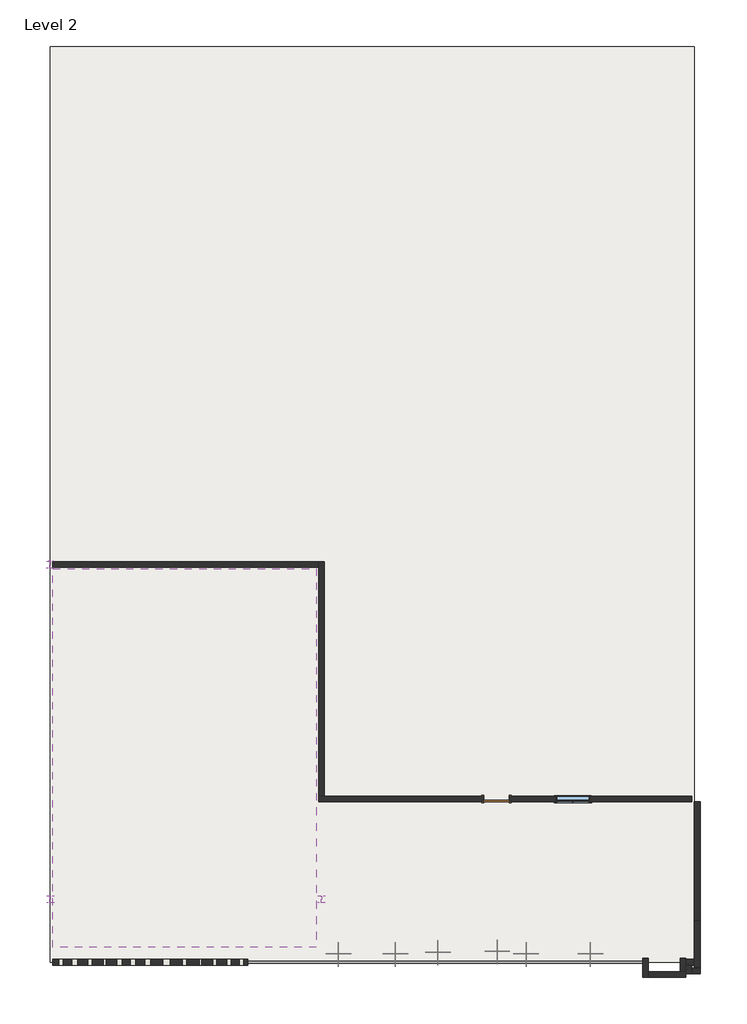
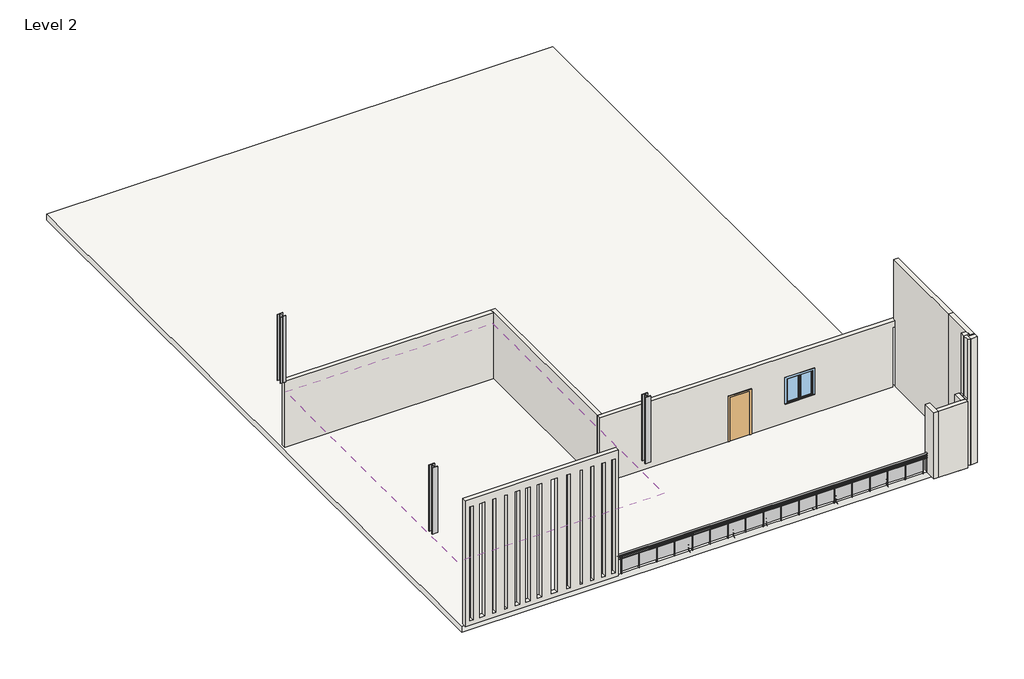
# One storey: 14 walls, 6 geographic elements, 3 columns, 1 covering, 1 door, 1 railing, 1 slab, 1 window.
"""IFC4 building model written with IfcOpenShell, lengths in millimetres."""

from ifc_helpers import new_model, si_unit, point, frame, origin, place, context, project, spatial, polyline, ellipse_curve, trimmed, outline, extrude, faceted_brep, transform, mapped, element, save
from ifc_brep_helpers import plane_surface, extruded_surface, advanced_brep
from components import w_shapes_column_w10x49_28d960f7, door_54dd4da4, rpc_plant_tropical_agave_1_5_93a2a214, window_0862ab64

model = new_model("IFC4")

# Units and contexts
model_context = context("Model", 3, world=origin())
ifc_project = project(units=[si_unit("LENGTHUNIT", "METRE", prefix="MILLI")], contexts=[model_context])

# Site, building, storey
site = spatial("IfcSite", under=ifc_project)
building = spatial("IfcBuilding", under=site)
storey = spatial("IfcBuildingStorey", under=building, Name="Level 2", Elevation=3200.4)

# Columns
placement = place(None, origin())
w_shapes_column_w10x49_shape = w_shapes_column_w10x49_28d960f7(model_context)
element("IfcColumn", 1, ObjectType="W Shapes-Column : W10X49", at=placement, inside=storey, context=model_context, shape_type="MappedRepresentation", body=[
    mapped(w_shapes_column_w10x49_shape, transform((-18401.1950104, -14607.7898918, 0.0), x_axis=(1.0, 0.0, 0.0), y_axis=(0.0, 1.0, 0.0), z_axis=(0.0, 0.0, 1.0))),
])
element("IfcColumn", 2, ObjectType="W Shapes-Column : W10X49", at=placement, inside=storey, context=model_context, shape_type="MappedRepresentation", body=[
    mapped(w_shapes_column_w10x49_shape, transform((-18401.1950104, -2573.393541, 0.0), x_axis=(1.0, 0.0, 0.0), y_axis=(0.0, 1.0, 0.0), z_axis=(0.0, 0.0, 1.0))),
])
element("IfcColumn", 3, ObjectType="W Shapes-Column : W10X49", at=placement, inside=storey, context=model_context, shape_type="MappedRepresentation", body=[
    mapped(w_shapes_column_w10x49_shape, transform((-8647.5950104, -14607.7898918, 0.0), x_axis=(1.0, 0.0, 0.0), y_axis=(0.0, 1.0, 0.0), z_axis=(0.0, 0.0, 1.0))),
])

# Covering
element("IfcCovering", 4, ObjectType="2' x 4' ACT System", at=placement, inside=storey, context=model_context, shape_type="SweptSolid", body=[
    extrude(outline(polyline([(-8829.5340594, -2725.793541), (-8829.5340594, -11305.7898918), (-8829.5340594, -16334.9898918), (-18299.5950104, -16334.9898918), (-18299.5950104, -2725.793541), (-8829.5340594, -2725.793541)])), frame((0.0, 0.0, 5943.6), z_axis=(0.0, 0.0, 1.0), x_axis=(1.0, 0.0, 0.0)), (0.0, 0.0, 1.0), 57.15),
    extrude(outline(polyline([(4712.8049896, -11305.7898918), (4712.8049896, -16334.9898918), (-8545.9950104, -16334.9898918), (-8545.9950104, -11305.7898918), (4712.8049896, -11305.7898918)])), frame((0.0, 0.0, 5943.6), z_axis=(0.0, 0.0, 1.0), x_axis=(1.0, 0.0, 0.0)), (0.0, 0.0, 1.0), 57.15),
])

# Door
door_shape = door_54dd4da4(model_context)
element("IfcDoor", 5, ObjectType="Single-Flush : 36\" x 84\"", at=placement, inside=storey, context=model_context, shape_type="MappedRepresentation", body=[
    mapped(door_shape, transform((-2348.3950104, -11000.9898918, 3200.4), x_axis=(-1.0, 0.0, 0.0), y_axis=(0.0, -1.0, 0.0), z_axis=(0.0, 0.0, 1.0))),
])

# Geographic elements
rpc_plant_tropical_agave_1_5_shape = rpc_plant_tropical_agave_1_5_93a2a214(model_context)
element("IfcGeographicElement", 6, ObjectType="RPC Plant - Tropical : Agave - 1.5'", at=placement, inside=storey, context=model_context, shape_type="MappedRepresentation", body=[
    mapped(rpc_plant_tropical_agave_1_5_shape, transform((-8037.9950104, -16571.4958521, 3200.4), x_axis=(1.0, 0.0, 0.0), y_axis=(0.0, 1.0, 0.0), z_axis=(0.0, 0.0, 1.0))),
])
element("IfcGeographicElement", 7, ObjectType="RPC Plant - Tropical : Agave - 1.5'", at=placement, inside=storey, context=model_context, shape_type="MappedRepresentation", body=[
    mapped(rpc_plant_tropical_agave_1_5_shape, transform((1023.9459392, -16571.4958521, 3200.4), x_axis=(1.0, 0.0, 0.0), y_axis=(0.0, 1.0, 0.0), z_axis=(0.0, 0.0, 1.0))),
])
element("IfcGeographicElement", 8, ObjectType="RPC Plant - Tropical : Agave - 1.5'", at=placement, inside=storey, context=model_context, shape_type="MappedRepresentation", body=[
    mapped(rpc_plant_tropical_agave_1_5_shape, transform((-1287.4540608, -16571.4958521, 3200.4), x_axis=(1.0, 0.0, 0.0), y_axis=(0.0, 1.0, 0.0), z_axis=(0.0, 0.0, 1.0))),
])
element("IfcGeographicElement", 9, ObjectType="RPC Plant - Tropical : Agave - 1.5'", at=placement, inside=storey, context=model_context, shape_type="MappedRepresentation", body=[
    mapped(rpc_plant_tropical_agave_1_5_shape, transform((-4462.4540608, -16512.2981542, 3200.4), x_axis=(1.0, 0.0, 0.0), y_axis=(0.0, 1.0, 0.0), z_axis=(0.0, 0.0, 1.0))),
])
element("IfcGeographicElement", 10, ObjectType="RPC Plant - Tropical : Agave - 1.5'", at=placement, inside=storey, context=model_context, shape_type="MappedRepresentation", body=[
    mapped(rpc_plant_tropical_agave_1_5_shape, transform((-5986.4540608, -16571.4958521, 3200.4), x_axis=(1.0, 0.0, 0.0), y_axis=(0.0, 1.0, 0.0), z_axis=(0.0, 0.0, 1.0))),
])
element("IfcGeographicElement", 11, ObjectType="RPC Plant - Tropical : Agave - 1.5'", at=placement, inside=storey, context=model_context, shape_type="MappedRepresentation", body=[
    mapped(rpc_plant_tropical_agave_1_5_shape, transform((-2328.8540608, -16476.9736509, 3200.4), x_axis=(1.0, 0.0, 0.0), y_axis=(0.0, 1.0, 0.0), z_axis=(0.0, 0.0, 1.0))),
])

# Railing
element("IfcRailing", 12, ObjectType="Glass Panel - Bottom Fill", at=placement, inside=storey, context=model_context, shape_type="SolidModel", body=[
    advanced_brep(
    [(-11289.1950104, -16830.2898918, 4114.8), (-11289.1950104, -16906.4898918, 4114.8), (2903.5459392, -16830.2898918, 4114.8), (2903.5459392, -16906.4898918, 4114.8)],
    [
        (0, 1, ellipse_curve(frame((-11289.1950104, -16868.3898918, 4114.8), z_axis=(-1.0, 0.0, 0.0), x_axis=(0.0, -1.0, 0.0)), 38.1, 28.575)),
        (1, 0, ellipse_curve(frame((-11289.1950104, -16868.3898918, 4114.8), z_axis=(-1.0, 0.0, 0.0), x_axis=(0.0, -1.0, 0.0)), 38.1, 28.575)),
        (2, 3, ellipse_curve(frame((2903.5459392, -16868.3898918, 4114.8), z_axis=(1.0, 0.0, 0.0), x_axis=(0.0, -1.0, 0.0)), 38.1, 28.575)),
        (3, 2, ellipse_curve(frame((2903.5459392, -16868.3898918, 4114.8), z_axis=(1.0, 0.0, 0.0), x_axis=(0.0, -1.0, 0.0)), 38.1, 28.575)),
        (0, 2),
        (3, 1),
    ],
    [
        plane_surface(frame((-11289.1950104, -16868.3898918, 4114.8), z_axis=(-1.0, 0.0, 0.0), x_axis=(0.0, 1.0, 0.0))),
        plane_surface(frame((2903.5459392, -16868.3898918, 4114.8), z_axis=(1.0, 0.0, 0.0), x_axis=(0.0, 1.0, 0.0))),
        extruded_surface(trimmed(ellipse_curve(frame((2903.5459392, -16868.3898918, 4114.8), z_axis=(-1.0, 0.0, 0.0), x_axis=(0.0, -1.0, 0.0)), 38.1, 28.575), [point((2903.5459392, -16830.2898918, 4114.8))], [point((2903.5459392, -16906.4898918, 4114.8))], True, "CARTESIAN"), (-14192.7409496, 0.0, 0.0), 14192.7409496),
        extruded_surface(trimmed(ellipse_curve(frame((2903.5459392, -16868.3898918, 4114.8), z_axis=(-1.0, 0.0, 0.0), x_axis=(0.0, -1.0, 0.0)), 38.1, 28.575), [point((2903.5459392, -16906.4898918, 4114.8))], [point((2903.5459392, -16830.2898918, 4114.8))], True, "CARTESIAN"), (-14192.7409496, 0.0, 0.0), 14192.7409496),
    ],
    [
        (0, [[1, 2]]),
        (1, [[3, 4]]),
        (2, [[-1, 5, -4, 6]]),
        (3, [[-2, -6, -3, -5]]),
    ],
),
    extrude(outline(polyline([(-11289.1950104, -16881.0898918), (-11289.1950104, -16855.6898918), (2903.5459392, -16855.6898918), (2903.5459392, -16881.0898918), (-11289.1950104, -16881.0898918)])), frame((0.0, 0.0, 4000.5), z_axis=(0.0, 0.0, 1.0), x_axis=(1.0, 0.0, 0.0)), (0.0, 0.0, 1.0), 25.4),
    extrude(outline(polyline([(-11289.1950104, -16881.0898918), (-11289.1950104, -16855.6898918), (2903.5459392, -16855.6898918), (2903.5459392, -16881.0898918), (-11289.1950104, -16881.0898918)])), frame((0.0, 0.0, 3898.9), z_axis=(0.0, 0.0, 1.0), x_axis=(1.0, 0.0, 0.0)), (0.0, 0.0, 1.0), 25.4),
    extrude(outline(polyline([(2709.6254644, -16893.7898918), (2709.6254644, -16842.9898918), (2722.3254644, -16842.9898918), (2722.3254644, -16893.7898918), (2709.6254644, -16893.7898918)])), frame((0.0, 0.0, 3200.4), z_axis=(0.0, 0.0, 1.0), x_axis=(1.0, 0.0, 0.0)), (0.0, 0.0, 1.0), 885.6788223),
    extrude(outline(polyline([(1903.1754644, -16861.8547348), (2715.9754644, -16861.8547348), (2715.9754644, -16868.2047348), (1903.1754644, -16868.2047348), (1903.1754644, -16861.8547348)])), frame((0.0, 0.0, 3302.0), z_axis=(0.0, 0.0, 1.0), x_axis=(1.0, 0.0, 0.0)), (0.0, 0.0, 1.0), 596.9),
    extrude(outline(polyline([(1896.8254644, -16893.7898918), (1896.8254644, -16842.9898918), (1909.5254644, -16842.9898918), (1909.5254644, -16893.7898918), (1896.8254644, -16893.7898918)])), frame((0.0, 0.0, 3200.4), z_axis=(0.0, 0.0, 1.0), x_axis=(1.0, 0.0, 0.0)), (0.0, 0.0, 1.0), 885.6788223),
    extrude(outline(polyline([(1090.3754644, -16861.8547348), (1903.1754644, -16861.8547348), (1903.1754644, -16868.2047348), (1090.3754644, -16868.2047348), (1090.3754644, -16861.8547348)])), frame((0.0, 0.0, 3302.0), z_axis=(0.0, 0.0, 1.0), x_axis=(1.0, 0.0, 0.0)), (0.0, 0.0, 1.0), 596.9),
    extrude(outline(polyline([(1084.0254644, -16893.7898918), (1084.0254644, -16842.9898918), (1096.7254644, -16842.9898918), (1096.7254644, -16893.7898918), (1084.0254644, -16893.7898918)])), frame((0.0, 0.0, 3200.4), z_axis=(0.0, 0.0, 1.0), x_axis=(1.0, 0.0, 0.0)), (0.0, 0.0, 1.0), 885.6788223),
    extrude(outline(polyline([(277.5754644, -16861.8547348), (1090.3754644, -16861.8547348), (1090.3754644, -16868.2047348), (277.5754644, -16868.2047348), (277.5754644, -16861.8547348)])), frame((0.0, 0.0, 3302.0), z_axis=(0.0, 0.0, 1.0), x_axis=(1.0, 0.0, 0.0)), (0.0, 0.0, 1.0), 596.9),
    extrude(outline(polyline([(271.2254644, -16893.7898918), (271.2254644, -16842.9898918), (283.9254644, -16842.9898918), (283.9254644, -16893.7898918), (271.2254644, -16893.7898918)])), frame((0.0, 0.0, 3200.4), z_axis=(0.0, 0.0, 1.0), x_axis=(1.0, 0.0, 0.0)), (0.0, 0.0, 1.0), 885.6788223),
    extrude(outline(polyline([(-535.2245356, -16861.8547348), (277.5754644, -16861.8547348), (277.5754644, -16868.2047348), (-535.2245356, -16868.2047348), (-535.2245356, -16861.8547348)])), frame((0.0, 0.0, 3302.0), z_axis=(0.0, 0.0, 1.0), x_axis=(1.0, 0.0, 0.0)), (0.0, 0.0, 1.0), 596.9),
    extrude(outline(polyline([(-541.5745356, -16893.7898918), (-541.5745356, -16842.9898918), (-528.8745356, -16842.9898918), (-528.8745356, -16893.7898918), (-541.5745356, -16893.7898918)])), frame((0.0, 0.0, 3200.4), z_axis=(0.0, 0.0, 1.0), x_axis=(1.0, 0.0, 0.0)), (0.0, 0.0, 1.0), 885.6788223),
    extrude(outline(polyline([(-1348.0245356, -16861.8547348), (-535.2245356, -16861.8547348), (-535.2245356, -16868.2047348), (-1348.0245356, -16868.2047348), (-1348.0245356, -16861.8547348)])), frame((0.0, 0.0, 3302.0), z_axis=(0.0, 0.0, 1.0), x_axis=(1.0, 0.0, 0.0)), (0.0, 0.0, 1.0), 596.9),
    extrude(outline(polyline([(-1354.3745356, -16893.7898918), (-1354.3745356, -16842.9898918), (-1341.6745356, -16842.9898918), (-1341.6745356, -16893.7898918), (-1354.3745356, -16893.7898918)])), frame((0.0, 0.0, 3200.4), z_axis=(0.0, 0.0, 1.0), x_axis=(1.0, 0.0, 0.0)), (0.0, 0.0, 1.0), 885.6788223),
    extrude(outline(polyline([(-2160.8245356, -16861.8547348), (-1348.0245356, -16861.8547348), (-1348.0245356, -16868.2047348), (-2160.8245356, -16868.2047348), (-2160.8245356, -16861.8547348)])), frame((0.0, 0.0, 3302.0), z_axis=(0.0, 0.0, 1.0), x_axis=(1.0, 0.0, 0.0)), (0.0, 0.0, 1.0), 596.9),
    extrude(outline(polyline([(-2167.1745356, -16893.7898918), (-2167.1745356, -16842.9898918), (-2154.4745356, -16842.9898918), (-2154.4745356, -16893.7898918), (-2167.1745356, -16893.7898918)])), frame((0.0, 0.0, 3200.4), z_axis=(0.0, 0.0, 1.0), x_axis=(1.0, 0.0, 0.0)), (0.0, 0.0, 1.0), 885.6788223),
    extrude(outline(polyline([(-2973.6245356, -16861.8547348), (-2160.8245356, -16861.8547348), (-2160.8245356, -16868.2047348), (-2973.6245356, -16868.2047348), (-2973.6245356, -16861.8547348)])), frame((0.0, 0.0, 3302.0), z_axis=(0.0, 0.0, 1.0), x_axis=(1.0, 0.0, 0.0)), (0.0, 0.0, 1.0), 596.9),
    extrude(outline(polyline([(-2979.9745356, -16893.7898918), (-2979.9745356, -16842.9898918), (-2967.2745356, -16842.9898918), (-2967.2745356, -16893.7898918), (-2979.9745356, -16893.7898918)])), frame((0.0, 0.0, 3200.4), z_axis=(0.0, 0.0, 1.0), x_axis=(1.0, 0.0, 0.0)), (0.0, 0.0, 1.0), 885.6788223),
    extrude(outline(polyline([(-3786.4245356, -16861.8547348), (-2973.6245356, -16861.8547348), (-2973.6245356, -16868.2047348), (-3786.4245356, -16868.2047348), (-3786.4245356, -16861.8547348)])), frame((0.0, 0.0, 3302.0), z_axis=(0.0, 0.0, 1.0), x_axis=(1.0, 0.0, 0.0)), (0.0, 0.0, 1.0), 596.9),
    extrude(outline(polyline([(-3792.7745356, -16893.7898918), (-3792.7745356, -16842.9898918), (-3780.0745356, -16842.9898918), (-3780.0745356, -16893.7898918), (-3792.7745356, -16893.7898918)])), frame((0.0, 0.0, 3200.4), z_axis=(0.0, 0.0, 1.0), x_axis=(1.0, 0.0, 0.0)), (0.0, 0.0, 1.0), 885.6788223),
    extrude(outline(polyline([(-4599.2245356, -16861.8547348), (-3786.4245356, -16861.8547348), (-3786.4245356, -16868.2047348), (-4599.2245356, -16868.2047348), (-4599.2245356, -16861.8547348)])), frame((0.0, 0.0, 3302.0), z_axis=(0.0, 0.0, 1.0), x_axis=(1.0, 0.0, 0.0)), (0.0, 0.0, 1.0), 596.9),
    extrude(outline(polyline([(-4605.5745356, -16893.7898918), (-4605.5745356, -16842.9898918), (-4592.8745356, -16842.9898918), (-4592.8745356, -16893.7898918), (-4605.5745356, -16893.7898918)])), frame((0.0, 0.0, 3200.4), z_axis=(0.0, 0.0, 1.0), x_axis=(1.0, 0.0, 0.0)), (0.0, 0.0, 1.0), 885.6788223),
    extrude(outline(polyline([(-5412.0245356, -16861.8547348), (-4599.2245356, -16861.8547348), (-4599.2245356, -16868.2047348), (-5412.0245356, -16868.2047348), (-5412.0245356, -16861.8547348)])), frame((0.0, 0.0, 3302.0), z_axis=(0.0, 0.0, 1.0), x_axis=(1.0, 0.0, 0.0)), (0.0, 0.0, 1.0), 596.9),
    extrude(outline(polyline([(-5418.3745356, -16893.7898918), (-5418.3745356, -16842.9898918), (-5405.6745356, -16842.9898918), (-5405.6745356, -16893.7898918), (-5418.3745356, -16893.7898918)])), frame((0.0, 0.0, 3200.4), z_axis=(0.0, 0.0, 1.0), x_axis=(1.0, 0.0, 0.0)), (0.0, 0.0, 1.0), 885.6788223),
    extrude(outline(polyline([(-6224.8245356, -16861.8547348), (-5412.0245356, -16861.8547348), (-5412.0245356, -16868.2047348), (-6224.8245356, -16868.2047348), (-6224.8245356, -16861.8547348)])), frame((0.0, 0.0, 3302.0), z_axis=(0.0, 0.0, 1.0), x_axis=(1.0, 0.0, 0.0)), (0.0, 0.0, 1.0), 596.9),
    extrude(outline(polyline([(-6231.1745356, -16893.7898918), (-6231.1745356, -16842.9898918), (-6218.4745356, -16842.9898918), (-6218.4745356, -16893.7898918), (-6231.1745356, -16893.7898918)])), frame((0.0, 0.0, 3200.4), z_axis=(0.0, 0.0, 1.0), x_axis=(1.0, 0.0, 0.0)), (0.0, 0.0, 1.0), 885.6788223),
    extrude(outline(polyline([(-7037.6245356, -16861.8547348), (-6224.8245356, -16861.8547348), (-6224.8245356, -16868.2047348), (-7037.6245356, -16868.2047348), (-7037.6245356, -16861.8547348)])), frame((0.0, 0.0, 3302.0), z_axis=(0.0, 0.0, 1.0), x_axis=(1.0, 0.0, 0.0)), (0.0, 0.0, 1.0), 596.9),
    extrude(outline(polyline([(-7043.9745356, -16893.7898918), (-7043.9745356, -16842.9898918), (-7031.2745356, -16842.9898918), (-7031.2745356, -16893.7898918), (-7043.9745356, -16893.7898918)])), frame((0.0, 0.0, 3200.4), z_axis=(0.0, 0.0, 1.0), x_axis=(1.0, 0.0, 0.0)), (0.0, 0.0, 1.0), 885.6788223),
    extrude(outline(polyline([(-7850.4245356, -16861.8547348), (-7037.6245356, -16861.8547348), (-7037.6245356, -16868.2047348), (-7850.4245356, -16868.2047348), (-7850.4245356, -16861.8547348)])), frame((0.0, 0.0, 3302.0), z_axis=(0.0, 0.0, 1.0), x_axis=(1.0, 0.0, 0.0)), (0.0, 0.0, 1.0), 596.9),
    extrude(outline(polyline([(-7856.7745356, -16893.7898918), (-7856.7745356, -16842.9898918), (-7844.0745356, -16842.9898918), (-7844.0745356, -16893.7898918), (-7856.7745356, -16893.7898918)])), frame((0.0, 0.0, 3200.4), z_axis=(0.0, 0.0, 1.0), x_axis=(1.0, 0.0, 0.0)), (0.0, 0.0, 1.0), 885.6788223),
    extrude(outline(polyline([(-8663.2245356, -16861.8547348), (-7850.4245356, -16861.8547348), (-7850.4245356, -16868.2047348), (-8663.2245356, -16868.2047348), (-8663.2245356, -16861.8547348)])), frame((0.0, 0.0, 3302.0), z_axis=(0.0, 0.0, 1.0), x_axis=(1.0, 0.0, 0.0)), (0.0, 0.0, 1.0), 596.9),
    extrude(outline(polyline([(-8669.5745356, -16893.7898918), (-8669.5745356, -16842.9898918), (-8656.8745356, -16842.9898918), (-8656.8745356, -16893.7898918), (-8669.5745356, -16893.7898918)])), frame((0.0, 0.0, 3200.4), z_axis=(0.0, 0.0, 1.0), x_axis=(1.0, 0.0, 0.0)), (0.0, 0.0, 1.0), 885.6788223),
    extrude(outline(polyline([(-9476.0245356, -16861.8547348), (-8663.2245356, -16861.8547348), (-8663.2245356, -16868.2047348), (-9476.0245356, -16868.2047348), (-9476.0245356, -16861.8547348)])), frame((0.0, 0.0, 3302.0), z_axis=(0.0, 0.0, 1.0), x_axis=(1.0, 0.0, 0.0)), (0.0, 0.0, 1.0), 596.9),
    extrude(outline(polyline([(-9482.3745356, -16893.7898918), (-9482.3745356, -16842.9898918), (-9469.6745356, -16842.9898918), (-9469.6745356, -16893.7898918), (-9482.3745356, -16893.7898918)])), frame((0.0, 0.0, 3200.4), z_axis=(0.0, 0.0, 1.0), x_axis=(1.0, 0.0, 0.0)), (0.0, 0.0, 1.0), 885.6788223),
    extrude(outline(polyline([(-10288.8245356, -16861.8547348), (-9476.0245356, -16861.8547348), (-9476.0245356, -16868.2047348), (-10288.8245356, -16868.2047348), (-10288.8245356, -16861.8547348)])), frame((0.0, 0.0, 3302.0), z_axis=(0.0, 0.0, 1.0), x_axis=(1.0, 0.0, 0.0)), (0.0, 0.0, 1.0), 596.9),
    extrude(outline(polyline([(-10295.1745356, -16893.7898918), (-10295.1745356, -16842.9898918), (-10282.4745356, -16842.9898918), (-10282.4745356, -16893.7898918), (-10295.1745356, -16893.7898918)])), frame((0.0, 0.0, 3200.4), z_axis=(0.0, 0.0, 1.0), x_axis=(1.0, 0.0, 0.0)), (0.0, 0.0, 1.0), 885.6788223),
    extrude(outline(polyline([(-11101.6245356, -16861.8547348), (-10288.8245356, -16861.8547348), (-10288.8245356, -16868.2047348), (-11101.6245356, -16868.2047348), (-11101.6245356, -16861.8547348)])), frame((0.0, 0.0, 3302.0), z_axis=(0.0, 0.0, 1.0), x_axis=(1.0, 0.0, 0.0)), (0.0, 0.0, 1.0), 596.9),
    extrude(outline(polyline([(-11107.9745356, -16893.7898918), (-11107.9745356, -16842.9898918), (-11095.2745356, -16842.9898918), (-11095.2745356, -16893.7898918), (-11107.9745356, -16893.7898918)])), frame((0.0, 0.0, 3200.4), z_axis=(0.0, 0.0, 1.0), x_axis=(1.0, 0.0, 0.0)), (0.0, 0.0, 1.0), 885.6788223),
    extrude(outline(polyline([(2890.8459392, -16877.9148918), (2890.8459392, -16858.8648918), (2909.8959392, -16858.8648918), (2909.8959392, -16877.9148918), (2890.8459392, -16877.9148918)])), frame((0.0, 0.0, 3200.4), z_axis=(0.0, 0.0, 1.0), x_axis=(1.0, 0.0, 0.0)), (0.0, 0.0, 1.0), 885.6788223),
    extrude(outline(polyline([(-11295.5450104, -16877.9148918), (-11295.5450104, -16858.8648918), (-11276.4950104, -16858.8648918), (-11276.4950104, -16877.9148918), (-11295.5450104, -16877.9148918)])), frame((0.0, 0.0, 3200.4), z_axis=(0.0, 0.0, 1.0), x_axis=(1.0, 0.0, 0.0)), (0.0, 0.0, 1.0), 885.6788223),
])

# Slab
element("IfcSlab", 13, ObjectType="Generic - 12\"", at=placement, inside=storey, context=model_context, shape_type="SweptSolid", body=[
    extrude(outline(polyline([(4763.6049896, 16050.0101082), (4763.6049896, -16868.3898918), (-18401.1950104, -16868.3898918), (-18401.1950104, 16050.0101082), (4763.6049896, 16050.0101082)])), frame((0.0, 0.0, 2895.6), z_axis=(0.0, 0.0, 1.0), x_axis=(1.0, 0.0, 0.0)), (0.0, 0.0, 1.0), 304.8),
])

# Walls
element("IfcWall", 14, at=placement, inside=storey, context=model_context, shape_type="Brep", body=[
    faceted_brep([(-2805.5950104, -10899.3898918, 5334.0), (-2805.5950104, -10899.3898918, 3200.4), (-8545.9950104, -10899.3898918, 3200.4), (-8749.1950104, -10899.3898918, 3200.4), (-8749.1950104, -10899.3898918, 6400.8), (-8545.9950104, -10899.3898918, 6400.8), (4966.8049896, -10899.3898918, 6400.8), (4966.8049896, -10899.3898918, 6096.0), (4662.0049896, -10899.3898918, 6096.0), (4662.0049896, -10899.3898918, 3200.4), (-1891.1950104, -10899.3898918, 3200.4), (-1891.1950104, -10899.3898918, 5334.0), (-214.7950104, -10899.3898918, 5334.0), (-214.7950104, -10899.3898918, 4114.8), (1004.4049896, -10899.3898918, 4114.8), (1004.4049896, -10899.3898918, 5334.0), (-8749.1950104, -11102.5898918, 3200.4), (-2805.5950104, -11102.5898918, 3200.4), (-2805.5950104, -11102.5898918, 5334.0), (-1891.1950104, -11102.5898918, 5334.0), (-1891.1950104, -11102.5898918, 3200.4), (4662.0049896, -11102.5898918, 3200.4), (4662.0049896, -11102.5898918, 6096.0), (4865.2049896, -11102.5898918, 6096.0), (4966.8049896, -11102.5898918, 6096.0), (4966.8049896, -11102.5898918, 6400.8), (4763.6049896, -11102.5898918, 6400.8), (-8749.1950104, -11102.5898918, 6400.8), (-214.7950104, -11102.5898918, 5334.0), (1004.4049896, -11102.5898918, 5334.0), (1004.4049896, -11102.5898918, 4114.8), (-214.7950104, -11102.5898918, 4114.8), (4966.8049896, -11000.9898918, 6400.8)], [[[0, 1, 2, 3, 4, 5, 6, 7, 8, 9, 10, 11], [12, 13, 14, 15]], [[16, 17, 18, 19, 20, 21, 22, 23, 24, 25, 26, 27], [28, 29, 30, 31]], [[10, 9, 21, 20]], [[3, 2, 1, 17, 16]], [[6, 5, 4, 27, 26, 25, 32]], [[4, 3, 16, 27]], [[7, 24, 23, 22, 8]], [[9, 8, 22, 21]], [[7, 6, 32, 25, 24]], [[13, 12, 28, 31]], [[14, 13, 31, 30]], [[15, 14, 30, 29]], [[12, 15, 29, 28]], [[18, 17, 1, 0]], [[19, 18, 0, 11]], [[20, 19, 11, 10]]]),
])
element("IfcWall", 15, at=placement, inside=storey, context=model_context, shape_type="Brep", body=[
    faceted_brep([(-18299.5950104, -16969.9898918, 3200.4), (-11289.1950104, -16969.9898918, 3200.4), (-11289.1950104, -16969.9898918, 9296.4), (-18299.5950104, -16969.9898918, 9296.4), (-18299.5950104, -16969.9898918, 6096.0), (-17936.4224264, -16969.9898918, 8919.5623487), (-17936.4224264, -16969.9898918, 3405.5276447), (-18088.8224264, -16969.9898918, 3405.5276447), (-18088.8224264, -16969.9898918, 8919.5623487), (-17404.6011344, -16969.9898918, 8919.5623487), (-17404.6011344, -16969.9898918, 3405.5276447), (-17628.2888645, -16969.9898918, 3405.5276447), (-17628.2888645, -16969.9898918, 8919.5623487), (-16891.4351653, -16969.9898918, 8919.5623487), (-16891.4351653, -16969.9898918, 3405.5276447), (-17049.3323866, -16969.9898918, 3405.5276447), (-17049.3323866, -16969.9898918, 8919.5623487), (-16378.2691963, -16969.9898918, 8919.5623487), (-16378.2691963, -16969.9898918, 3405.5276447), (-16496.6921122, -16969.9898918, 3405.5276447), (-16496.6921122, -16969.9898918, 8919.5623487), (-15812.4708202, -16969.9898918, 8919.5623487), (-15812.4708202, -16969.9898918, 3405.5276447), (-16009.8423468, -16969.9898918, 3405.5276447), (-16009.8423468, -16969.9898918, 8919.5623487), (-15522.9925813, -16969.9898918, 8919.5623487), (-15312.4629529, -16969.9898918, 8919.5623487), (-15312.4629529, -16969.9898918, 3405.5276447), (-15522.9925813, -16969.9898918, 3405.5276447), (-14786.1388821, -16969.9898918, 8919.5623487), (-14786.1388821, -16969.9898918, 3405.5276447), (-14996.6685105, -16969.9898918, 3405.5276447), (-14996.6685105, -16969.9898918, 8919.5623487), (-14088.7594883, -16969.9898918, 8919.5623487), (-14088.7594883, -16969.9898918, 3405.5276447), (-14351.9215237, -16969.9898918, 3405.5276447), (-14351.9215237, -16969.9898918, 8919.5623487), (-13496.6449087, -16969.9898918, 8919.5623487), (-13496.6449087, -16969.9898918, 3405.5276447), (-13654.5421299, -16969.9898918, 3405.5276447), (-13654.5421299, -16969.9898918, 8919.5623487), (-12944.0046343, -16969.9898918, 8919.5623487), (-12944.0046343, -16969.9898918, 3405.5276447), (-13036.1113467, -16969.9898918, 3405.5276447), (-13036.1113467, -16969.9898918, 8919.5623487), (-12417.6805635, -16969.9898918, 8919.5623487), (-12417.6805635, -16969.9898918, 3405.5276447), (-12549.2615812, -16969.9898918, 3405.5276447), (-12549.2615812, -16969.9898918, 8919.5623487), (-11891.3564927, -16969.9898918, 8919.5623487), (-11891.3564927, -16969.9898918, 3405.5276447), (-12049.2537139, -16969.9898918, 3405.5276447), (-12049.2537139, -16969.9898918, 8919.5623487), (-11430.8229307, -16969.9898918, 8919.5623487), (-11430.8229307, -16969.9898918, 3405.5276447), (-11601.8782538, -16969.9898918, 3405.5276447), (-11601.8782538, -16969.9898918, 8919.5623487), (-18299.5950104, -16766.7898918, 3200.4), (-18299.5950104, -16766.7898918, 9296.4), (-11289.1950104, -16766.7898918, 9296.4), (-11289.1950104, -16766.7898918, 3200.4), (-17936.4224264, -16766.7898918, 8919.5623487), (-18088.8224264, -16766.7898918, 8919.5623487), (-18088.8224264, -16766.7898918, 3405.5276447), (-17936.4224264, -16766.7898918, 3405.5276447), (-17404.6011344, -16766.7898918, 8919.5623487), (-17628.2888645, -16766.7898918, 8919.5623487), (-17628.2888645, -16766.7898918, 3405.5276447), (-17404.6011344, -16766.7898918, 3405.5276447), (-16891.4351653, -16766.7898918, 8919.5623487), (-17049.3323866, -16766.7898918, 8919.5623487), (-17049.3323866, -16766.7898918, 3405.5276447), (-16891.4351653, -16766.7898918, 3405.5276447), (-16378.2691963, -16766.7898918, 8919.5623487), (-16496.6921122, -16766.7898918, 8919.5623487), (-16496.6921122, -16766.7898918, 3405.5276447), (-16378.2691963, -16766.7898918, 3405.5276447), (-15812.4708202, -16766.7898918, 8919.5623487), (-16009.8423468, -16766.7898918, 8919.5623487), (-16009.8423468, -16766.7898918, 3405.5276447), (-15812.4708202, -16766.7898918, 3405.5276447), (-15522.9925813, -16766.7898918, 8919.5623487), (-15522.9925813, -16766.7898918, 3405.5276447), (-15312.4629529, -16766.7898918, 3405.5276447), (-15312.4629529, -16766.7898918, 8919.5623487), (-14786.1388821, -16766.7898918, 8919.5623487), (-14996.6685105, -16766.7898918, 8919.5623487), (-14996.6685105, -16766.7898918, 3405.5276447), (-14786.1388821, -16766.7898918, 3405.5276447), (-14088.7594883, -16766.7898918, 8919.5623487), (-14351.9215237, -16766.7898918, 8919.5623487), (-14351.9215237, -16766.7898918, 3405.5276447), (-14088.7594883, -16766.7898918, 3405.5276447), (-13496.6449087, -16766.7898918, 8919.5623487), (-13654.5421299, -16766.7898918, 8919.5623487), (-13654.5421299, -16766.7898918, 3405.5276447), (-13496.6449087, -16766.7898918, 3405.5276447), (-12944.0046343, -16766.7898918, 8919.5623487), (-13036.1113467, -16766.7898918, 8919.5623487), (-13036.1113467, -16766.7898918, 3405.5276447), (-12944.0046343, -16766.7898918, 3405.5276447), (-12417.6805635, -16766.7898918, 8919.5623487), (-12549.2615812, -16766.7898918, 8919.5623487), (-12549.2615812, -16766.7898918, 3405.5276447), (-12417.6805635, -16766.7898918, 3405.5276447), (-11891.3564927, -16766.7898918, 8919.5623487), (-12049.2537139, -16766.7898918, 8919.5623487), (-12049.2537139, -16766.7898918, 3405.5276447), (-11891.3564927, -16766.7898918, 3405.5276447), (-11430.8229307, -16766.7898918, 8919.5623487), (-11601.8782538, -16766.7898918, 8919.5623487), (-11601.8782538, -16766.7898918, 3405.5276447), (-11430.8229307, -16766.7898918, 3405.5276447), (-18299.5950104, -16893.7898918, 3200.4)], [[[0, 1, 2, 3, 4], [5, 6, 7, 8], [9, 10, 11, 12], [13, 14, 15, 16], [17, 18, 19, 20], [21, 22, 23, 24], [25, 26, 27, 28], [29, 30, 31, 32], [33, 34, 35, 36], [37, 38, 39, 40], [41, 42, 43, 44], [45, 46, 47, 48], [49, 50, 51, 52], [53, 54, 55, 56]], [[57, 58, 59, 60], [61, 62, 63, 64], [65, 66, 67, 68], [69, 70, 71, 72], [73, 74, 75, 76], [77, 78, 79, 80], [81, 82, 83, 84], [85, 86, 87, 88], [89, 90, 91, 92], [93, 94, 95, 96], [97, 98, 99, 100], [101, 102, 103, 104], [105, 106, 107, 108], [109, 110, 111, 112]], [[0, 4, 3, 58, 57, 113]], [[1, 0, 113, 57, 60]], [[2, 1, 60, 59]], [[3, 2, 59, 58]], [[6, 5, 61, 64]], [[7, 6, 64, 63]], [[8, 7, 63, 62]], [[5, 8, 62, 61]], [[10, 9, 65, 68]], [[11, 10, 68, 67]], [[12, 11, 67, 66]], [[9, 12, 66, 65]], [[14, 13, 69, 72]], [[15, 14, 72, 71]], [[16, 15, 71, 70]], [[13, 16, 70, 69]], [[18, 17, 73, 76]], [[19, 18, 76, 75]], [[20, 19, 75, 74]], [[17, 20, 74, 73]], [[22, 21, 77, 80]], [[23, 22, 80, 79]], [[24, 23, 79, 78]], [[21, 24, 78, 77]], [[26, 25, 81, 84]], [[27, 26, 84, 83]], [[28, 27, 83, 82]], [[25, 28, 82, 81]], [[30, 29, 85, 88]], [[31, 30, 88, 87]], [[32, 31, 87, 86]], [[29, 32, 86, 85]], [[34, 33, 89, 92]], [[35, 34, 92, 91]], [[36, 35, 91, 90]], [[33, 36, 90, 89]], [[38, 37, 93, 96]], [[39, 38, 96, 95]], [[40, 39, 95, 94]], [[37, 40, 94, 93]], [[42, 41, 97, 100]], [[43, 42, 100, 99]], [[44, 43, 99, 98]], [[41, 44, 98, 97]], [[46, 45, 101, 104]], [[47, 46, 104, 103]], [[48, 47, 103, 102]], [[45, 48, 102, 101]], [[50, 49, 105, 108]], [[51, 50, 108, 107]], [[52, 51, 107, 106]], [[49, 52, 106, 105]], [[54, 53, 109, 112]], [[55, 54, 112, 111]], [[56, 55, 111, 110]], [[53, 56, 110, 109]]]),
])
element("IfcWall", 16, ObjectType="Generic - 8\"", at=placement, inside=storey, context=model_context, shape_type="Brep", body=[
    faceted_brep([(-8545.9950104, -10899.3898918, 3200.4), (-8545.9950104, -2471.793541, 3200.4), (-8545.9950104, -2471.793541, 6400.8), (-8545.9950104, -10899.3898918, 6400.8), (-8749.1950104, -10899.3898918, 3200.4), (-8749.1950104, -10899.3898918, 6400.8), (-8749.1950104, -2674.993541, 6400.8), (-8749.1950104, -2471.793541, 6400.8), (-8749.1950104, -2471.793541, 3200.4), (-8749.1950104, -2674.993541, 3200.4)], [[[0, 1, 2, 3]], [[4, 5, 6, 7, 8, 9]], [[1, 0, 4, 9, 8]], [[3, 2, 7, 6, 5]], [[0, 3, 5, 4]], [[2, 1, 8, 7]]]),
])
element("IfcWall", 17, ObjectType="Generic - 8\"", at=placement, inside=storey, context=model_context, shape_type="SweptSolid", body=[
    extrude(outline(polyline([(-18299.5950104, -2471.793541), (-8749.1950104, -2471.793541), (-8749.1950104, -2674.993541), (-18299.5950104, -2674.993541), (-18299.5950104, -2471.793541)])), frame((0.0, 0.0, 3200.4), z_axis=(0.0, 0.0, 1.0), x_axis=(1.0, 0.0, 0.0)), (0.0, 0.0, 1.0), 3200.4),
])
element("IfcWall", 18, ObjectType="Generic - 8\"", at=placement, inside=storey, context=model_context, shape_type="Brep", body=[
    faceted_brep([(4763.6049896, -11102.5898918, 3200.4), (4763.6049896, -17046.1898918, 3200.4), (4763.6049896, -17046.1898918, 9296.4), (4763.6049896, -11000.9898918, 9296.4), (4763.6049896, -11000.9898918, 6400.8), (4763.6049896, -11102.5898918, 6400.8), (4966.8049896, -11102.5898918, 3200.4), (4966.8049896, -11102.5898918, 6096.0), (4966.8049896, -11102.5898918, 6400.8), (4966.8049896, -11000.9898918, 6400.8), (4966.8049896, -11000.9898918, 9296.4), (4966.8049896, -17046.1898918, 9296.4), (4966.8049896, -17046.1898918, 3200.4), (4865.2049896, -11102.5898918, 3200.4), (4890.6049896, -11000.9898918, 6400.8), (4839.8049896, -11000.9898918, 6400.8)], [[[0, 1, 2, 3, 4, 5]], [[6, 7, 8, 9, 10, 11, 12]], [[1, 0, 13, 6, 12]], [[2, 1, 12, 11]], [[3, 2, 11, 10]], [[4, 3, 10, 9, 14, 15]], [[4, 15, 14, 9, 8, 5]], [[0, 5, 8, 7, 6, 13]]]),
])
element("IfcWall", 19, ObjectType="Generic - 8\"", at=placement, inside=storey, context=model_context, shape_type="SweptSolid", body=[
    extrude(outline(polyline([(4966.8049896, -15369.7898918), (4966.8049896, -17046.1898918), (4763.6049896, -17046.1898918), (4763.6049896, -15369.7898918), (4966.8049896, -15369.7898918)])), frame((0.0, 0.0, 3200.4), z_axis=(0.0, 0.0, 1.0), x_axis=(1.0, 0.0, 0.0)), (0.0, 0.0, 1.0), 6096.0),
])
element("IfcWall", 20, ObjectType="Generic - 8\"", at=placement, inside=storey, context=model_context, shape_type="Brep", body=[
    faceted_brep([(4454.4050598, -16969.9898918, 3200.4), (4657.6050598, -16969.9898918, 3200.4), (4763.6049896, -16969.9898918, 3200.4), (4763.6049896, -16969.9898918, 9296.4), (4657.6050598, -16969.9898918, 9296.4), (4528.1321681, -16969.9898918, 9296.4), (4528.1321681, -16969.9898918, 6400.8), (4454.4050598, -16969.9898918, 6400.8), (4454.4050598, -16766.7898918, 3200.4), (4454.4050598, -16766.7898918, 6400.8), (4528.1321681, -16766.7898918, 6400.8), (4528.1321681, -16766.7898918, 9296.4), (4763.6049896, -16766.7898918, 9296.4), (4763.6049896, -16766.7898918, 3200.4)], [[[0, 1, 2, 3, 4, 5, 6, 7]], [[8, 9, 10, 11, 12, 13]], [[2, 1, 0, 8, 13]], [[0, 7, 9, 8]], [[3, 2, 13, 12]], [[5, 4, 3, 12, 11]], [[5, 11, 10, 6]], [[7, 6, 10, 9]]]),
])
element("IfcWall", 21, ObjectType="Generic - 8\"", at=placement, inside=storey, context=model_context, shape_type="Brep", body=[
    faceted_brep([(4657.6050598, -17287.4954298, 3200.4), (4657.6050598, -17084.2954298, 3200.4), (4657.6050598, -16969.9898918, 3200.4), (4657.6050598, -16969.9898918, 9296.4), (4657.6050598, -17084.2954298, 9296.4), (4657.6050598, -17287.4954298, 9296.4), (4454.4050598, -17287.4954298, 3200.4), (4454.4050598, -17287.4954298, 6400.8), (4454.4050598, -16969.9898918, 6400.8), (4454.4050598, -16969.9898918, 3200.4), (4528.1321681, -17287.4954298, 9296.4), (4528.1321681, -17287.4954298, 6400.8), (4528.1321681, -16969.9898918, 6400.8), (4528.1321681, -16969.9898918, 9296.4)], [[[0, 1, 2, 3, 4, 5]], [[6, 7, 8, 9]], [[2, 1, 0, 6, 9]], [[0, 5, 10, 11, 7, 6]], [[3, 2, 9, 8, 12, 13]], [[5, 4, 3, 13, 10]], [[10, 13, 12, 11]], [[12, 8, 7, 11]]]),
])
element("IfcWall", 22, ObjectType="Generic - 8\"", at=placement, inside=storey, context=model_context, shape_type="Brep", body=[
    faceted_brep([(4966.8049896, -17084.2954298, 3200.4), (4763.6049896, -17084.2954298, 3200.4), (4657.6050598, -17084.2954298, 3200.4), (4657.6050598, -17084.2954298, 9296.4), (4763.6049896, -17084.2954298, 9296.4), (4966.8049896, -17084.2954298, 9296.4), (4966.8049896, -17287.4954298, 3200.4), (4966.8049896, -17287.4954298, 9296.4), (4657.6050598, -17287.4954298, 9296.4), (4657.6050598, -17287.4954298, 3200.4)], [[[0, 1, 2, 3, 4, 5]], [[6, 7, 8, 9]], [[2, 1, 0, 6, 9]], [[5, 4, 3, 8, 7]], [[0, 5, 7, 6]], [[3, 2, 9, 8]]]),
])
element("IfcWall", 23, ObjectType="Generic - 8\"", at=placement, inside=storey, context=model_context, shape_type="Brep", body=[
    faceted_brep([(4763.6049896, -16766.7898918, 3200.4), (4763.6049896, -16969.9898918, 3200.4), (4763.6049896, -17084.2954298, 3200.4), (4763.6049896, -17084.2954298, 9296.4), (4763.6049896, -16969.9898918, 9296.4), (4763.6049896, -16766.7898918, 9296.4), (4966.8049896, -16766.7898918, 3200.4), (4966.8049896, -16766.7898918, 9296.4), (4966.8049896, -17084.2954298, 9296.4), (4966.8049896, -17084.2954298, 3200.4)], [[[0, 1, 2, 3, 4, 5]], [[6, 7, 8, 9]], [[2, 1, 0, 6, 9]], [[5, 4, 3, 8, 7]], [[0, 5, 7, 6]], [[3, 2, 9, 8]]]),
])
element("IfcWall", 24, ObjectType="Generic - 8\"", at=placement, inside=storey, context=model_context, shape_type="Brep", body=[
    faceted_brep([(3106.7459392, -17415.097968, 3200.4), (3106.7459392, -17211.897968, 3200.4), (3106.7459392, -16729.297968, 3200.4), (3106.7459392, -16729.297968, 6400.8), (3106.7459392, -17211.897968, 6400.8), (3106.7459392, -17415.097968, 6400.8), (2903.5459392, -17415.097968, 3200.4), (2903.5459392, -17415.097968, 6400.8), (2903.5459392, -16729.297968, 6400.8), (2903.5459392, -16729.297968, 3200.4)], [[[0, 1, 2, 3, 4, 5]], [[6, 7, 8, 9]], [[2, 1, 0, 6, 9]], [[3, 2, 9, 8]], [[0, 5, 7, 6]], [[5, 4, 3, 8, 7]]]),
])
element("IfcWall", 25, ObjectType="Generic - 8\"", at=placement, inside=storey, context=model_context, shape_type="Brep", body=[
    faceted_brep([(4452.9459392, -17211.897968, 3200.4), (4249.7459392, -17211.897968, 3200.4), (3106.7459392, -17211.897968, 3200.4), (3106.7459392, -17211.897968, 6400.8), (4249.7459392, -17211.897968, 6400.8), (4452.9459392, -17211.897968, 6400.8), (4452.9459392, -17415.097968, 3200.4), (4452.9459392, -17415.097968, 6400.8), (3106.7459392, -17415.097968, 6400.8), (3106.7459392, -17415.097968, 3200.4)], [[[0, 1, 2, 3, 4, 5]], [[6, 7, 8, 9]], [[2, 1, 0, 6, 9]], [[0, 5, 7, 6]], [[3, 2, 9, 8]], [[5, 4, 3, 8, 7]]]),
])
element("IfcWall", 26, ObjectType="Generic - 8\"", at=placement, inside=storey, context=model_context, shape_type="SweptSolid", body=[
    extrude(outline(polyline([(4249.7459392, -17211.897968), (4249.7459392, -16729.297968), (4452.9459392, -16729.297968), (4452.9459392, -17211.897968), (4249.7459392, -17211.897968)])), frame((0.0, 0.0, 3200.4), z_axis=(0.0, 0.0, 1.0), x_axis=(1.0, 0.0, 0.0)), (0.0, 0.0, 1.0), 3200.4),
])
element("IfcWall", 27, ObjectType="Generic - 8\"", at=placement, inside=storey, context=model_context, shape_type="SweptSolid", body=[
    extrude(outline(polyline([(3106.7459392, -17211.897968), (4249.7459392, -17211.897968), (4249.7459392, -17415.097968), (3106.7459392, -17415.097968), (3106.7459392, -17211.897968)])), frame((0.0, 0.0, 3200.4), z_axis=(0.0, 0.0, 1.0), x_axis=(1.0, 0.0, 0.0)), (0.0, 0.0, 1.0), 3200.4),
])

# Window
window_shape = window_0862ab64(model_context)
element("IfcWindow", 28, ObjectType="Casement Dbl with Trim : 48\" x 48\"", at=placement, inside=storey, context=model_context, shape_type="MappedRepresentation", body=[
    mapped(window_shape, transform((394.8049896, -10981.9398918, 3200.4), x_axis=(-1.0, 0.0, 0.0), y_axis=(0.0, -1.0, 0.0), z_axis=(0.0, 0.0, 1.0))),
])

save(model, "model.ifc")

# Revit data of these elements
# Type "W Shapes-Column : W10X49"
#   Section Name Key = "W10x49"
#   Assembly Code = "B10"
#   Width = 10.000"
#   Web Thickness = 0.340"
#   Web Fillet = 0.500"
#   Warping Constant = 2070.00 in⁶
#   Torsional Moment of Inertia = 1.39 in⁴
#   Section Area = 14.40 in²
#   Plastic Modulus weak axis = 28.30 in³
#   Plastic Modulus strong axis = 60.40 in³
#   Perimeter = 58.50 ft²/ft
#   Nominal Weight = 49.00 lbf/ft
#   Moment of Inertia weak axis = 93.40 in⁴
#   Moment of Inertia strong axis = 272.00 in⁴
#   Height = 10.000"
#   Flange Thickness = 0.560"
#   Elastic Modulus weak axis = 18.70 in³
#   Elastic Modulus strong axis = 54.60 in³
#   Centroid Vertical = 5.000"
#   Centroid Horizontal = 5.000"
#   Structural Material [instance default] = Steel ASTM A992
#   Principal Axes Angle = 0
# Type "2' x 4' ACT System"
#   Assembly Code = "C3030210"
#   built-in parameter 1002203 = 1 (stored number, unit not read)
#   built-in parameter 1002202 = 1 (stored number, unit not read)
#   Layers, outside or top first: 0' - 1 5/8" "Default" (function 1); 0' - 0 5/8" "Acoustic Ceiling Tile 24 x 48" (function 5)
# Type "Single-Flush : 36\" x 84\""
#   Type Mark = "1"
#   Construction Type Id = "MDOOR"
#   Assembly Code = "C1020"
#   Analytic Construction = "Metal"
#   Thickness = 0' - 2"
#   Heat Transfer Coefficient (U) = 0.651978 BTU/(h·ft²·°F)
#   Height = 7' - 0"
#   Trim Projection Ext = 0' - 1"
#   Trim Projection Int = 0' - 1"
#   Trim Width = 0' - 3"
#   Width = 3' - 0"
#   Define Thermal Properties by = 1
#   Door Material = Door - Panel
#   Frame Material = Door - Frame
#   Visual Light Transmittance = 0
#   Solar Heat Gain Coefficient = 0
#   Function = (empty or 0)
#   Wall Closure = (empty or 0)
# Type "RPC Plant - Tropical : Agave - 1.5'"
#   built-in parameter 1005198 = "{2, 15},{39, RPC-16-G1GJ-63FX-7K5P-N000-ST1L-LVER-AU},{1, 0},{1, 0},{2, 13},{1, 8},{5, Color},{1, 0},{1, 0},{3, 0.8},{3, 0.8},{3, 0.8},{1, 8},{7, BBoxMin},{1, 0},{1, 0},{1, 0},{1, 0},{1, 0},{1, 8},{7, BBoxMax},{1, 0},{1, 0},{1, 0},{1, 0},{1, 0},{2, 11},{9, RPCTypeId},{1, 0},{1, 0},{39, RPC-16-G1GJ-63FX-7K5P-N000-ST1L-LVER-AU},{1, 6},{14, RPCPlantHeight},{1, 0},{1, 0},{3, 1.5},{2, 11},{7, keyword},{1, 0},{1, 0},{35, :RPCs:Plants [General]:Geometry:RPC},{2, 11},{8, category},{1, 0},{1, 0},{16, Plants [General]},{2, 11},{12, LocalizedUID},{1, 0},{1, 0},{5, Agave},{2, 14},{6, Height},{1, 0},{1, 0},{3, 1.5},{1, 2},{16, Cast Reflections},{1, 0},{1, 0},{1, 0},{1, 2},{12, Cast Shadows},{1, 0},{1, 0},{1, 1},{1, 2},{9, Lock View},{1, 0},{1, 0},{1, 0},{1, 4},{5, ViewC},{1, 0},{1, 0},{1, 0},{21, assetlibrary_base.fbx},{1, 5},"
#   built-in parameter 1005195 = "RPC-16-G1GJ-63FX-7K5P-N000-ST1L-LVER-AU"
#   Type Comments = "Agave"
#   Assembly Code = "G2050500"
#   Height = 1' - 6"
#   Default Elevation = 0
# Type "Glass Panel - Bottom Fill"
#   Assembly Code = "C2010400"
#   built-in parameter 1008612 = 0.0416667 (stored number, unit not read)
#   built-in parameter 1008611 = 0.0416667 (stored number, unit not read)
#   built-in parameter 1008609 = 0.333333 (stored number, unit not read)
#   built-in parameter 1008604 = 0.166667 (stored number, unit not read)
#   built-in parameter 1008603 = 0.166667 (stored number, unit not read)
#   Railing Height = 3' - 0"
#   built-in parameter 1008630 = 2
#   built-in parameter 1008610 = 2
#   built-in parameter 1008618 = Baluster - Square : 3/4"
# Type "Generic - 12\""
#   Assembly Code = "B1010"
#   Function = 0
#   Layers, outside or top first: 1' - 0" no material (function 1)
# Type
#   Assembly Code = "B2010"
#   Layers, outside or top first: 0' - 8" "Sash" (function 1)
# Type "Generic - 8\""
#   Assembly Code = "B2010"
#   Layers, outside or top first: 0' - 8" no material (function 1)
# Type "Casement Dbl with Trim : 48\" x 48\""
#   Type Mark = "19"
#   Construction Type Id = "GSP4R"
#   Assembly Code = "B2020100"
#   Analytic Construction = "1/8 in Pilkington single glazing"
#   Visual Light Transmittance = 0.9
#   Solar Heat Gain Coefficient = 0.78
#   Heat Transfer Coefficient (U) = 0.6496 BTU/(h·ft²·°F)
#   Height = 4' - 0"
#   Default Sill Height = 3' - 0"
#   Trim Projection - Ext. = 0' - 0 1/2"
#   Trim Projection - Int. = 0' - 0 3/4"
#   Trim Width - Exterior = 0' - 3 1/2"
#   Trim Width - Interior = 0' - 3 1/2"
#   Width = 4' - 0"
#   Window Inset = 0' - 0 3/4"
#   Define Thermal Properties by = 1
#   Glass Pane Material = Glass
#   Sash Material = Sash
#   Trim Exterior Material = Trim
#   Trim Interior Material = Trim
#   Wall Closure = (empty or 0)
# Elements 1, 2, 3 (IfcColumn, "W Shapes-Column : W10X49")
#   Structural Material = Steel ASTM A992
#   Phase Created = New Construction
#   Materials on its faces: "Steel ASTM A992"
# Element 4 (IfcCovering, "2' x 4' ACT System")
#   Height Offset From Level = 9' - 0"
#   Phase Created = New Construction
#   Materials on its faces: "Acoustic Ceiling Tile 24 x 48", "Default"
# Element 5 (IfcDoor, "Single-Flush : 36\" x 84\"")
#   Phase Created = New Construction
#   Materials on its faces: "Door - Frame", "Door - Panel"
# Elements 6, 7, 8, 9, 10, 11 (IfcGeographicElement, "RPC Plant - Tropical : Agave - 1.5'")
#   Phase Created = New Construction
# Element 12 (IfcRailing, "Glass Panel - Bottom Fill")
#   Phase Created = New Construction
#   Materials on its faces: "Glass"
# Element 13 (IfcSlab, "Generic - 12\"")
#   Height Offset From Level = 0' - 0"
#   Phase Created = New Construction
#   Materials on its faces: "Default Floor"
# Element 14 (IfcWall)
#   Top Offset = 0' - 0"
#   Base Offset = 0' - 0"
#   Unconnected Height = 10' - 6"
#   wall height = 10' - 6"
#   Phase Created = New Construction
#   Base Constraint = Level 2
#   Materials on its faces: "Sash", "Default Wall"
# Element 15 (IfcWall)
#   Top Offset = 0' - 0"
#   Base Offset = 0' - 0"
#   Unconnected Height = 20' - 0"
#   wall height = 20' - 0"
#   Phase Created = New Construction
#   Base Constraint = Level 2
#   Materials on its faces: "Sash"
# Elements 16, 17 (IfcWall, "Generic - 8\"")
#   Top Offset = 0' - 0"
#   Base Offset = 0' - 0"
#   Unconnected Height = 10' - 6"
#   wall height = 10' - 6"
#   Phase Created = New Construction
#   Base Constraint = Level 2
#   Materials on its faces: "Default Wall"
# Elements 18, 19, 20, 21, 22, 23, 24, 25, 26, 27 (IfcWall, "Generic - 8\"")
#   Top Offset = 0' - 0"
#   Base Offset = 0' - 0"
#   Unconnected Height = 20' - 0"
#   wall height = 20' - 0"
#   Phase Created = New Construction
#   Base Constraint = Level 2
#   Materials on its faces: "Default Wall"
# Element 28 (IfcWindow, "Casement Dbl with Trim : 48\" x 48\"")
#   Mark = "2"
#   Phase Created = New Construction
#   Materials on its faces: "Sash", "Trim", "Glass"
# Materials
#   "Steel ASTM A992": class "Metal", colour RGB 199 199 199, transparency 0, Description = "Structural steel 50ksi", Cost = 0
#   "Default": colour RGB 127 127 127, transparency 0
#   "Acoustic Ceiling Tile 24 x 48": class "Generic", colour RGB 229 229 229, transparency 0, Description = "Acoustic Ceiling Tile 24 x 48", Cost = 0
#   "Door - Panel": class "Wood", colour RGB 210 159 95, transparency 0
#   "Door - Frame": colour RGB 118 70 51, transparency 0
#   "Sash": class "Wood", colour RGB 255 255 255, transparency 0, Cost = 0
#   "Glass": class "Glass", colour RGB 0 128 192, transparency 0.75, Description = "Soda Lime Glass", Cost = 0
#   "Trim": class "Wood", colour RGB 224 178 126, transparency 0
#   "Default Floor": colour RGB 128 128 128, transparency 0
#   "Default Wall": colour RGB 128 128 128, transparency 0
